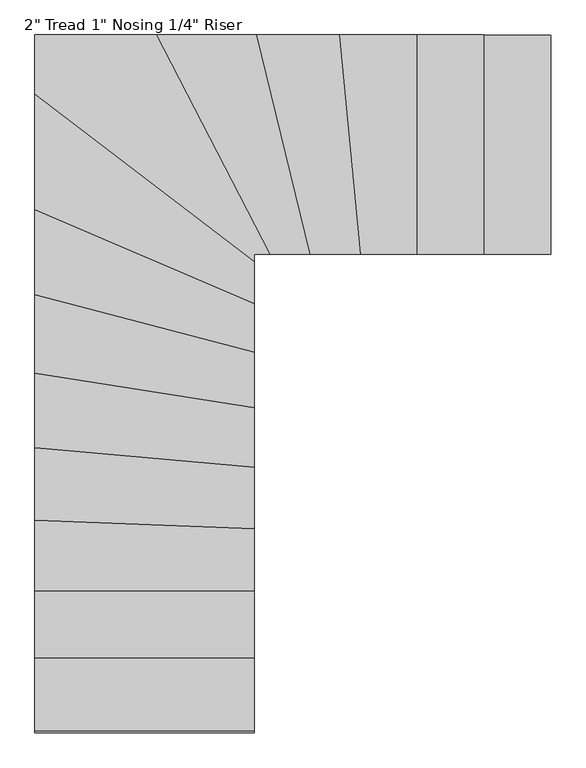
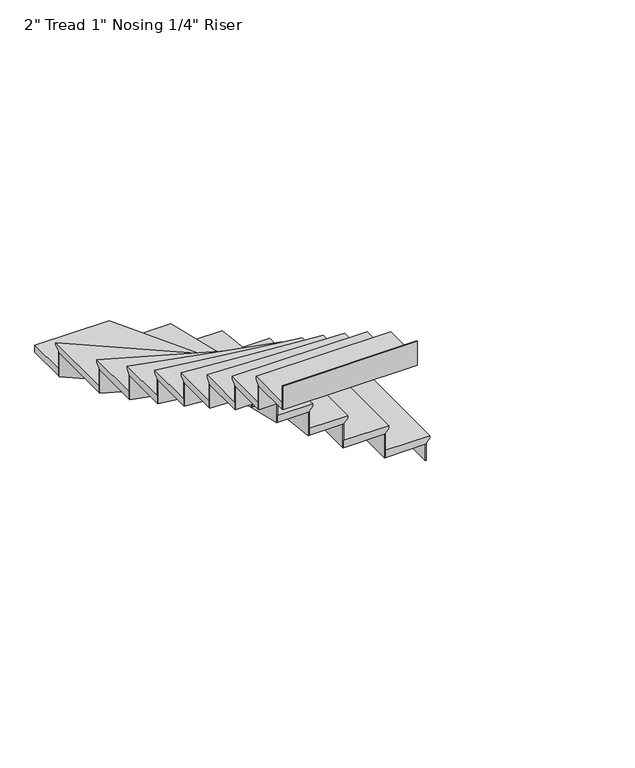
"""IFC4 building model written with IfcOpenShell, lengths in millimetres: stair flight geometry."""

from ifc_helpers import new_model, si_unit, origin, place, context, project, spatial, faceted_brep, source, transform, mapped, element, save


def stair_flight_393df7a1(model_context):
    return source(origin(), model_context, "Body", "Brep", [
        faceted_brep([(-4892.6027934, 5526.7691167, 319.6166667), (-4892.6027934, 5526.7691167, 338.6666667), (-4892.6027934, 4612.3691167, 338.6666667), (-4892.6027934, 4612.3691167, 319.6166667), (-4918.0027934, 5526.7691167, 294.2166667), (-4918.0027934, 4612.3691167, 294.2166667), (-5197.4027934, 5526.7691167, 338.6666667), (-5197.4027934, 4612.3691167, 338.6666667), (-4918.0027934, 4612.3691167, 287.8666667), (-5197.4027934, 4612.3691167, 287.8666667), (-5197.4027934, 5526.7691167, 287.8666667), (-4918.0027934, 5526.7691167, 287.8666667)], [[[0, 1, 2, 3]], [[4, 0, 3, 5]], [[2, 1, 6, 7]], [[8, 9, 10, 11]], [[2, 7, 9, 8, 5, 3]], [[8, 11, 4, 5]], [[6, 1, 0, 4, 11, 10]], [[7, 6, 10, 9]]]),
        faceted_brep([(-4918.0027934, 5526.7691167, 287.8666667), (-4918.0027934, 5526.7691167, 169.3333333), (-4924.3527934, 5526.7691167, 169.3333333), (-4924.3527934, 5526.7691167, 287.8666667), (-4918.0027934, 4612.3691167, 287.8666667), (-4924.3527934, 4612.3691167, 287.8666667), (-4924.3527934, 4612.3691167, 169.3333333), (-4918.0027934, 4612.3691167, 169.3333333)], [[[0, 1, 2, 3]], [[4, 5, 6, 7]], [[1, 0, 4, 7]], [[2, 1, 7, 6]], [[3, 2, 6, 5]], [[0, 3, 5, 4]]]),
        faceted_brep([(-5197.4027934, 5526.7691167, 457.2), (-5197.4027934, 5526.7691167, 287.8666667), (-5203.7527934, 5526.7691167, 287.8666667), (-5203.7527934, 5526.7691167, 457.2), (-5197.4027934, 4612.3691167, 457.2), (-5203.7527934, 4612.3691167, 457.2), (-5203.7527934, 4612.3691167, 287.8666667), (-5197.4027934, 4612.3691167, 287.8666667)], [[[0, 1, 2, 3]], [[4, 5, 6, 7]], [[1, 0, 4, 7]], [[2, 1, 7, 6]], [[3, 2, 6, 5]], [[0, 3, 5, 4]]]),
        faceted_brep([(-5172.0027934, 4612.3691167, 508.0), (-5172.0027934, 5526.7691167, 508.0), (-5476.8027934, 5526.7691167, 508.0), (-5476.8027934, 4612.3691167, 508.0), (-5197.4027934, 4612.3691167, 457.2), (-5476.8027934, 4612.3691167, 457.2), (-5476.8027934, 5526.7691167, 457.2), (-5197.4027934, 5526.7691167, 457.2), (-5197.4027934, 4612.3691167, 463.55), (-5172.0027934, 4612.3691167, 488.95), (-5197.4027934, 5526.7691167, 463.55), (-5172.0027934, 5526.7691167, 488.95)], [[[0, 1, 2, 3]], [[4, 5, 6, 7]], [[0, 3, 5, 4, 8, 9]], [[4, 7, 10, 8]], [[2, 1, 11, 10, 7, 6]], [[3, 2, 6, 5]], [[11, 1, 0, 9]], [[10, 11, 9, 8]]]),
        faceted_brep([(-5476.8027934, 5526.7691167, 626.5333333), (-5476.8027934, 5526.7691167, 457.2), (-5483.1527934, 5526.7691167, 457.2), (-5483.1527934, 5526.7691167, 626.5333333), (-5476.8027934, 4612.3691167, 626.5333333), (-5483.1527934, 4612.3691167, 626.5333333), (-5483.1527934, 4612.3691167, 457.2), (-5476.8027934, 4612.3691167, 457.2)], [[[0, 1, 2, 3]], [[4, 5, 6, 7]], [[1, 0, 4, 7]], [[2, 1, 7, 6]], [[3, 2, 6, 5]], [[0, 3, 5, 4]]]),
        faceted_brep([(-5451.4027934, 4612.3691167, 677.3333333), (-5451.4027934, 5526.7691167, 677.3333333), (-5800.1202782, 5526.7691167, 677.3333333), (-5712.5179034, 4612.3691167, 677.3333333), (-5476.8027934, 4612.3691167, 626.5333333), (-5712.5179034, 4612.3691167, 626.5333333), (-5800.1202782, 5526.7691167, 626.5333333), (-5476.8027934, 5526.7691167, 626.5333333), (-5476.8027934, 4612.3691167, 632.8833333), (-5451.4027934, 4612.3691167, 658.2833333), (-5476.8027934, 5526.7691167, 632.8833333), (-5451.4027934, 5526.7691167, 658.2833333)], [[[0, 1, 2, 3]], [[4, 5, 6, 7]], [[0, 3, 5, 4, 8, 9]], [[4, 7, 10, 8]], [[2, 1, 11, 10, 7, 6]], [[3, 2, 6, 5]], [[11, 1, 0, 9]], [[10, 11, 9, 8]]]),
        faceted_brep([(-5800.1202782, 5526.7691167, 795.8666667), (-5800.1202782, 5526.7691167, 626.5333333), (-5806.4993526, 5526.7691167, 626.5333333), (-5806.4993526, 5526.7691167, 795.8666667), (-5712.5179034, 4612.3691167, 795.8666667), (-5718.8969778, 4612.3691167, 795.8666667), (-5718.8969778, 4612.3691167, 626.5333333), (-5712.5179034, 4612.3691167, 626.5333333)], [[[0, 1, 2, 3]], [[4, 5, 6, 7]], [[1, 0, 4, 7]], [[2, 1, 7, 6]], [[3, 2, 6, 5]], [[0, 3, 5, 4]]]),
        faceted_brep([(-5687.0016061, 4612.3691167, 846.6666667), (-5774.6039808, 5526.7691167, 846.6666667), (-6148.4006476, 5526.7691167, 846.6666667), (-5924.3082092, 4612.3691167, 846.6666667), (-5712.5179034, 4612.3691167, 795.8666667), (-5924.3082092, 4612.3691167, 795.8666667), (-6148.4006476, 5526.7691167, 795.8666667), (-5800.1202782, 5526.7691167, 795.8666667), (-5712.5179034, 4612.3691167, 802.2166667), (-5687.0016061, 4612.3691167, 827.6166667), (-5800.1202782, 5526.7691167, 802.2166667), (-5774.6039808, 5526.7691167, 827.6166667)], [[[0, 1, 2, 3]], [[4, 5, 6, 7]], [[0, 3, 5, 4, 8, 9]], [[4, 7, 10, 8]], [[2, 1, 11, 10, 7, 6]], [[3, 2, 6, 5]], [[11, 1, 0, 9]], [[10, 11, 9, 8]]]),
        faceted_brep([(-6148.4006476, 5526.7691167, 965.2), (-6148.4006476, 5526.7691167, 795.8666667), (-6154.9385563, 5526.7691167, 795.8666667), (-6154.9385563, 5526.7691167, 965.2), (-5924.3082092, 4612.3691167, 965.2), (-5930.8461179, 4612.3691167, 965.2), (-5930.8461179, 4612.3691167, 795.8666667), (-5924.3082092, 4612.3691167, 795.8666667)], [[[0, 1, 2, 3]], [[4, 5, 6, 7]], [[1, 0, 4, 7]], [[2, 1, 7, 6]], [[3, 2, 6, 5]], [[0, 3, 5, 4]]]),
        faceted_brep([(-5898.1565743, 4612.3691167, 1016.0), (-6122.2490126, 5526.7691167, 1016.0), (-6568.0298157, 5526.7691167, 1016.0), (-6094.5265481, 4612.3691167, 1016.0), (-5924.3082092, 4612.3691167, 965.2), (-6094.5265481, 4612.3691167, 965.2), (-6568.0298157, 5526.7691167, 965.2), (-6148.4006476, 5526.7691167, 965.2), (-5924.3082092, 4612.3691167, 971.55), (-5898.1565743, 4612.3691167, 996.95), (-6148.4006476, 5526.7691167, 971.55), (-6122.2490126, 5526.7691167, 996.95)], [[[0, 1, 2, 3]], [[4, 5, 6, 7]], [[0, 3, 5, 4, 8, 9]], [[4, 7, 10, 8]], [[2, 1, 11, 10, 7, 6]], [[3, 2, 6, 5]], [[11, 1, 0, 9]], [[10, 11, 9, 8]]]),
        faceted_brep([(-6568.0298157, 5526.7691167, 1134.5333333), (-6568.0298157, 5526.7691167, 965.2), (-6575.1806808, 5526.7691167, 965.2), (-6575.1806808, 5526.7691167, 1134.5333333), (-6094.5265481, 4612.3691167, 1134.5333333), (-6101.6774133, 4612.3691167, 1134.5333333), (-6101.6774133, 4612.3691167, 965.2), (-6094.5265481, 4612.3691167, 965.2)], [[[0, 1, 2, 3]], [[4, 5, 6, 7]], [[1, 0, 4, 7]], [[2, 1, 7, 6]], [[3, 2, 6, 5]], [[0, 3, 5, 4]]]),
        faceted_brep([(-6130.7957152, 4549.1663649, 1185.3333333), (-6130.7957152, 4612.3691167, 1185.3333333), (-6065.9230877, 4612.3691167, 1185.3333333), (-6539.4263552, 5526.7691167, 1185.3333333), (-7045.1957152, 5526.7691167, 1185.3333333), (-7045.1957152, 5248.0321012, 1185.3333333), (-6130.7957152, 4612.3691167, 1134.5333333), (-6130.7957152, 4549.1663649, 1134.5333333), (-7045.1957152, 5248.0321012, 1134.5333333), (-7045.1957152, 5526.7691167, 1134.5333333), (-6568.0298157, 5526.7691167, 1134.5333333), (-6094.5265481, 4612.3691167, 1134.5333333), (-6568.0298157, 5526.7691167, 1140.8833333), (-6094.5265481, 4612.3691167, 1140.8833333), (-6539.4263552, 5526.7691167, 1166.2833333), (-6065.9230877, 4612.3691167, 1166.2833333)], [[[0, 1, 2, 3, 4, 5]], [[6, 7, 8, 9, 10, 11]], [[1, 0, 7, 6]], [[11, 10, 12, 13]], [[4, 3, 14, 12, 10, 9]], [[0, 5, 8, 7]], [[14, 3, 2, 15]], [[12, 14, 15, 13]], [[2, 1, 6, 11, 13, 15]], [[5, 4, 9, 8]]]),
        faceted_brep([(-7045.1957152, 5248.0321012, 1303.8666667), (-7045.1957152, 5248.0321012, 1134.5333333), (-7045.1957152, 5240.039831, 1134.5333333), (-7045.1957152, 5240.039831, 1303.8666667), (-6130.7957152, 4549.1663649, 1303.8666667), (-6130.7957152, 4541.1740947, 1303.8666667), (-6130.7957152, 4541.1740947, 1134.5333333), (-6130.7957152, 4549.1663649, 1134.5333333)], [[[0, 1, 2, 3]], [[4, 5, 6, 7]], [[1, 0, 4, 7]], [[2, 1, 7, 6]], [[3, 2, 6, 5]], [[0, 3, 5, 4]]]),
        faceted_brep([(-6130.7957152, 4581.1354457, 1354.6666667), (-7045.1957152, 5280.001182, 1354.6666667), (-7045.1957152, 4770.0134963, 1354.6666667), (-6130.7957152, 4378.7251797, 1354.6666667), (-6130.7957152, 4549.1663649, 1303.8666667), (-6130.7957152, 4378.7251797, 1303.8666667), (-7045.1957152, 4770.0134963, 1303.8666667), (-7045.1957152, 5248.0321012, 1303.8666667), (-6130.7957152, 4549.1663649, 1310.2166667), (-6130.7957152, 4581.1354457, 1335.6166667), (-7045.1957152, 5248.0321012, 1310.2166667), (-7045.1957152, 5280.001182, 1335.6166667)], [[[0, 1, 2, 3]], [[4, 5, 6, 7]], [[0, 3, 5, 4, 8, 9]], [[4, 7, 10, 8]], [[2, 1, 11, 10, 7, 6]], [[3, 2, 6, 5]], [[11, 1, 0, 9]], [[10, 11, 9, 8]]]),
        faceted_brep([(-7045.1957152, 4770.0134963, 1473.2), (-7045.1957152, 4770.0134963, 1303.8666667), (-7045.1957152, 4763.1065352, 1303.8666667), (-7045.1957152, 4763.1065352, 1473.2), (-6130.7957152, 4378.7251797, 1473.2), (-6130.7957152, 4371.8182187, 1473.2), (-6130.7957152, 4371.8182187, 1303.8666667), (-6130.7957152, 4378.7251797, 1303.8666667)], [[[0, 1, 2, 3]], [[4, 5, 6, 7]], [[1, 0, 4, 7]], [[2, 1, 7, 6]], [[3, 2, 6, 5]], [[0, 3, 5, 4]]]),
        faceted_brep([(-6130.7957152, 4406.3530238, 1524.0), (-7045.1957152, 4797.6413403, 1524.0), (-7045.1957152, 4415.9634084, 1524.0), (-6130.7957152, 4176.7209832, 1524.0), (-6130.7957152, 4378.7251797, 1473.2), (-6130.7957152, 4176.7209832, 1473.2), (-7045.1957152, 4415.9634084, 1473.2), (-7045.1957152, 4770.0134963, 1473.2), (-6130.7957152, 4378.7251797, 1479.55), (-6130.7957152, 4406.3530238, 1504.95), (-7045.1957152, 4770.0134963, 1479.55), (-7045.1957152, 4797.6413403, 1504.95)], [[[0, 1, 2, 3]], [[4, 5, 6, 7]], [[0, 3, 5, 4, 8, 9]], [[4, 7, 10, 8]], [[2, 1, 11, 10, 7, 6]], [[3, 2, 6, 5]], [[11, 1, 0, 9]], [[10, 11, 9, 8]]]),
        faceted_brep([(-7045.1957152, 4415.9634084, 1642.5333333), (-7045.1957152, 4415.9634084, 1473.2), (-7045.1957152, 4409.3996618, 1473.2), (-7045.1957152, 4409.3996618, 1642.5333333), (-6130.7957152, 4176.7209832, 1642.5333333), (-6130.7957152, 4170.1572366, 1642.5333333), (-6130.7957152, 4170.1572366, 1473.2), (-6130.7957152, 4176.7209832, 1473.2)], [[[0, 1, 2, 3]], [[4, 5, 6, 7]], [[1, 0, 4, 7]], [[2, 1, 7, 6]], [[3, 2, 6, 5]], [[0, 3, 5, 4]]]),
        faceted_brep([(-6130.7957152, 4202.9759694, 1693.3333333), (-7045.1957152, 4442.2183946, 1693.3333333), (-7045.1957152, 4090.08094, 1693.3333333), (-6130.7957152, 3944.8769125, 1693.3333333), (-6130.7957152, 4176.7209832, 1642.5333333), (-6130.7957152, 3944.8769125, 1642.5333333), (-7045.1957152, 4090.08094, 1642.5333333), (-7045.1957152, 4415.9634084, 1642.5333333), (-6130.7957152, 4176.7209832, 1648.8833333), (-6130.7957152, 4202.9759694, 1674.2833333), (-7045.1957152, 4415.9634084, 1648.8833333), (-7045.1957152, 4442.2183946, 1674.2833333)], [[[0, 1, 2, 3]], [[4, 5, 6, 7]], [[0, 3, 5, 4, 8, 9]], [[4, 7, 10, 8]], [[2, 1, 11, 10, 7, 6]], [[3, 2, 6, 5]], [[11, 1, 0, 9]], [[10, 11, 9, 8]]]),
        faceted_brep([(-7045.1957152, 4090.08094, 1811.8666667), (-7045.1957152, 4090.08094, 1642.5333333), (-7045.1957152, 4083.6513761, 1642.5333333), (-7045.1957152, 4083.6513761, 1811.8666667), (-6130.7957152, 3944.8769125, 1811.8666667), (-6130.7957152, 3938.4473486, 1811.8666667), (-6130.7957152, 3938.4473486, 1642.5333333), (-6130.7957152, 3944.8769125, 1642.5333333)], [[[0, 1, 2, 3]], [[4, 5, 6, 7]], [[1, 0, 4, 7]], [[2, 1, 7, 6]], [[3, 2, 6, 5]], [[0, 3, 5, 4]]]),
        faceted_brep([(-6130.7957152, 3970.5951683, 1862.6666667), (-7045.1957152, 4115.7991958, 1862.6666667), (-7045.1957152, 3778.9445524, 1862.6666667), (-6130.7957152, 3697.6494409, 1862.6666667), (-6130.7957152, 3944.8769125, 1811.8666667), (-6130.7957152, 3697.6494409, 1811.8666667), (-7045.1957152, 3778.9445524, 1811.8666667), (-7045.1957152, 4090.08094, 1811.8666667), (-6130.7957152, 3944.8769125, 1818.2166667), (-6130.7957152, 3970.5951683, 1843.6166667), (-7045.1957152, 4090.08094, 1818.2166667), (-7045.1957152, 4115.7991958, 1843.6166667)], [[[0, 1, 2, 3]], [[4, 5, 6, 7]], [[0, 3, 5, 4, 8, 9]], [[4, 7, 10, 8]], [[2, 1, 11, 10, 7, 6]], [[3, 2, 6, 5]], [[11, 1, 0, 9]], [[10, 11, 9, 8]]]),
        faceted_brep([(-7045.1957152, 3778.9445524, 1981.2), (-7045.1957152, 3778.9445524, 1811.8666667), (-7045.1957152, 3772.569506, 1811.8666667), (-7045.1957152, 3772.569506, 1981.2), (-6130.7957152, 3697.6494409, 1981.2), (-6130.7957152, 3691.2743945, 1981.2), (-6130.7957152, 3691.2743945, 1811.8666667), (-6130.7957152, 3697.6494409, 1811.8666667)], [[[0, 1, 2, 3]], [[4, 5, 6, 7]], [[1, 0, 4, 7]], [[2, 1, 7, 6]], [[3, 2, 6, 5]], [[0, 3, 5, 4]]]),
        faceted_brep([(-6130.7957152, 3723.1496263, 2032.0), (-7045.1957152, 3804.4447378, 2032.0), (-7045.1957152, 3476.4960567, 2032.0), (-6130.7957152, 3441.4610333, 2032.0), (-6130.7957152, 3697.6494409, 1981.2), (-6130.7957152, 3441.4610333, 1981.2), (-7045.1957152, 3476.4960567, 1981.2), (-7045.1957152, 3778.9445524, 1981.2), (-6130.7957152, 3697.6494409, 1987.55), (-6130.7957152, 3723.1496263, 2012.95), (-7045.1957152, 3778.9445524, 1987.55), (-7045.1957152, 3804.4447378, 2012.95)], [[[0, 1, 2, 3]], [[4, 5, 6, 7]], [[0, 3, 5, 4, 8, 9]], [[4, 7, 10, 8]], [[2, 1, 11, 10, 7, 6]], [[3, 2, 6, 5]], [[11, 1, 0, 9]], [[10, 11, 9, 8]]]),
        faceted_brep([(-7045.1957152, 3476.4960567, 2150.5333333), (-7045.1957152, 3476.4960567, 1981.2), (-7045.1957152, 3470.1413975, 1981.2), (-7045.1957152, 3470.1413975, 2150.5333333), (-6130.7957152, 3441.4610333, 2150.5333333), (-6130.7957152, 3435.106374, 2150.5333333), (-6130.7957152, 3435.106374, 1981.2), (-6130.7957152, 3441.4610333, 1981.2)], [[[0, 1, 2, 3]], [[4, 5, 6, 7]], [[1, 0, 4, 7]], [[2, 1, 7, 6]], [[3, 2, 6, 5]], [[0, 3, 5, 4]]]),
        faceted_brep([(-6130.7957152, 3466.8796703, 2201.3333333), (-7045.1957152, 3501.9146937, 2201.3333333), (-7045.1957152, 3179.597182, 2201.3333333), (-6130.7957152, 3179.597182, 2201.3333333), (-6130.7957152, 3441.4610333, 2150.5333333), (-6130.7957152, 3179.597182, 2150.5333333), (-7045.1957152, 3179.597182, 2150.5333333), (-7045.1957152, 3476.4960567, 2150.5333333), (-6130.7957152, 3441.4610333, 2156.8833333), (-6130.7957152, 3466.8796703, 2182.2833333), (-7045.1957152, 3476.4960567, 2156.8833333), (-7045.1957152, 3501.9146937, 2182.2833333)], [[[0, 1, 2, 3]], [[4, 5, 6, 7]], [[0, 3, 5, 4, 8, 9]], [[4, 7, 10, 8]], [[2, 1, 11, 10, 7, 6]], [[3, 2, 6, 5]], [[11, 1, 0, 9]], [[10, 11, 9, 8]]]),
        faceted_brep([(-7045.1957152, 3179.597182, 2319.8666667), (-7045.1957152, 3179.597182, 2150.5333333), (-7045.1957152, 3173.247182, 2150.5333333), (-7045.1957152, 3173.247182, 2319.8666667), (-6130.7957152, 3179.597182, 2319.8666667), (-6130.7957152, 3173.247182, 2319.8666667), (-6130.7957152, 3173.247182, 2150.5333333), (-6130.7957152, 3179.597182, 2150.5333333)], [[[0, 1, 2, 3]], [[4, 5, 6, 7]], [[1, 0, 4, 7]], [[2, 1, 7, 6]], [[3, 2, 6, 5]], [[0, 3, 5, 4]]]),
        faceted_brep([(-6130.7957152, 3204.997182, 2370.6666667), (-7045.1957152, 3204.997182, 2370.6666667), (-7045.1957152, 2900.197182, 2370.6666667), (-6130.7957152, 2900.197182, 2370.6666667), (-6130.7957152, 3179.597182, 2319.8666667), (-6130.7957152, 2900.197182, 2319.8666667), (-7045.1957152, 2900.197182, 2319.8666667), (-7045.1957152, 3179.597182, 2319.8666667), (-6130.7957152, 3179.597182, 2326.2166667), (-6130.7957152, 3204.997182, 2351.6166667), (-7045.1957152, 3179.597182, 2326.2166667), (-7045.1957152, 3204.997182, 2351.6166667)], [[[0, 1, 2, 3]], [[4, 5, 6, 7]], [[0, 3, 5, 4, 8, 9]], [[4, 7, 10, 8]], [[2, 1, 11, 10, 7, 6]], [[3, 2, 6, 5]], [[11, 1, 0, 9]], [[10, 11, 9, 8]]]),
        faceted_brep([(-7045.1957152, 2900.197182, 2489.2), (-7045.1957152, 2900.197182, 2319.8666667), (-7045.1957152, 2893.847182, 2319.8666667), (-7045.1957152, 2893.847182, 2489.2), (-6130.7957152, 2900.197182, 2489.2), (-6130.7957152, 2893.847182, 2489.2), (-6130.7957152, 2893.847182, 2319.8666667), (-6130.7957152, 2900.197182, 2319.8666667)], [[[0, 1, 2, 3]], [[4, 5, 6, 7]], [[1, 0, 4, 7]], [[2, 1, 7, 6]], [[3, 2, 6, 5]], [[0, 3, 5, 4]]]),
        faceted_brep([(-7045.1957152, 2620.797182, 2658.5333333), (-7045.1957152, 2620.797182, 2489.2), (-7045.1957152, 2614.447182, 2489.2), (-7045.1957152, 2614.447182, 2658.5333333), (-6130.7957152, 2620.797182, 2658.5333333), (-6130.7957152, 2614.447182, 2658.5333333), (-6130.7957152, 2614.447182, 2489.2), (-6130.7957152, 2620.797182, 2489.2)], [[[0, 1, 2, 3]], [[4, 5, 6, 7]], [[1, 0, 4, 7]], [[2, 1, 7, 6]], [[3, 2, 6, 5]], [[0, 3, 5, 4]]]),
        faceted_brep([(-6130.7957152, 2925.597182, 2540.0), (-7045.1957152, 2925.597182, 2540.0), (-7045.1957152, 2620.797182, 2540.0), (-6130.7957152, 2620.797182, 2540.0), (-6130.7957152, 2900.197182, 2489.2), (-6130.7957152, 2620.797182, 2489.2), (-7045.1957152, 2620.797182, 2489.2), (-7045.1957152, 2900.197182, 2489.2), (-6130.7957152, 2900.197182, 2495.55), (-6130.7957152, 2925.597182, 2520.95), (-7045.1957152, 2900.197182, 2495.55), (-7045.1957152, 2925.597182, 2520.95)], [[[0, 1, 2, 3]], [[4, 5, 6, 7]], [[0, 3, 5, 4, 8, 9]], [[4, 7, 10, 8]], [[2, 1, 11, 10, 7, 6]], [[3, 2, 6, 5]], [[11, 1, 0, 9]], [[10, 11, 9, 8]]]),
    ])


if __name__ == "__main__":
    model = new_model("IFC4")
    model_context = context("Model", 3, world=origin())
    ifc_project = project(units=[si_unit("LENGTHUNIT", "METRE", prefix="MILLI")], contexts=[model_context])
    site = spatial("IfcSite", under=ifc_project)
    building = spatial("IfcBuilding", under=site)
    placement = place(None, origin())
    stair_flight_shape = stair_flight_393df7a1(model_context)
    element("IfcStairFlight", 1, ObjectType="2\" Tread 1\" Nosing 1/4\" Riser", at=placement, inside=building, context=model_context, shape_type="MappedRepresentation", body=[
        mapped(stair_flight_shape, transform((0.0, 0.0, 0.0), x_axis=(1.0, 0.0, 0.0), y_axis=(0.0, 1.0, 0.0), z_axis=(0.0, 0.0, 1.0))),
    ])
    save(model, "model.ifc")
